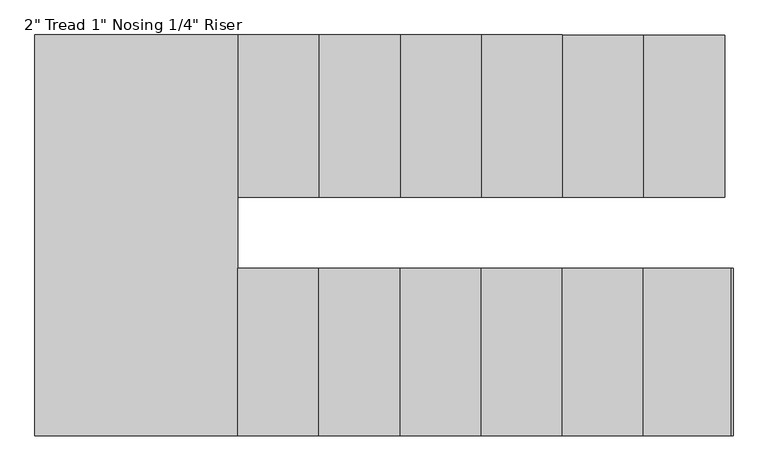
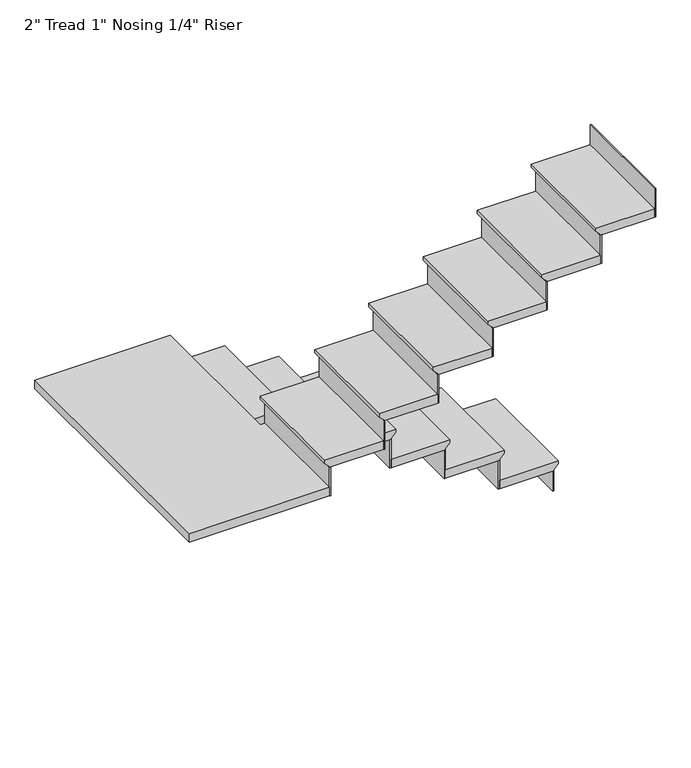
"""IFC4 building model written with IfcOpenShell, lengths in millimetres: stair flight geometry."""

from ifc_helpers import new_model, si_unit, origin, place, context, project, spatial, faceted_brep, source, transform, mapped, element, save


def stair_flight_411a5c89(model_context):
    return source(origin(), model_context, "Body", "Brep", [
        faceted_brep([(-2968.8120155, -2170.0065691, 12951.8833333), (-2968.8120155, -2170.0065691, 12970.9333333), (-2968.8120155, -2779.6065691, 12970.9333333), (-2968.8120155, -2779.6065691, 12951.8833333), (-2994.2120155, -2170.0065691, 12926.4833333), (-2994.2120155, -2779.6065691, 12926.4833333), (-3299.0120155, -2170.0065691, 12970.9333333), (-3299.0120155, -2779.6065691, 12970.9333333), (-2994.2120155, -2779.6065691, 12920.1333333), (-3299.0120155, -2779.6065691, 12920.1333333), (-3299.0120155, -2170.0065691, 12920.1333333), (-2994.2120155, -2170.0065691, 12920.1333333)], [[[0, 1, 2, 3]], [[4, 0, 3, 5]], [[2, 1, 6, 7]], [[8, 9, 10, 11]], [[2, 7, 9, 8, 5, 3]], [[8, 11, 4, 5]], [[6, 1, 0, 4, 11, 10]], [[7, 6, 10, 9]]]),
        faceted_brep([(-2994.2120155, -2170.0065691, 12920.1333333), (-2994.2120155, -2170.0065691, 12801.6), (-3000.5620155, -2170.0065691, 12801.6), (-3000.5620155, -2170.0065691, 12920.1333333), (-2994.2120155, -2779.6065691, 12920.1333333), (-3000.5620155, -2779.6065691, 12920.1333333), (-3000.5620155, -2779.6065691, 12801.6), (-2994.2120155, -2779.6065691, 12801.6)], [[[0, 1, 2, 3]], [[4, 5, 6, 7]], [[1, 0, 4, 7]], [[2, 1, 7, 6]], [[3, 2, 6, 5]], [[0, 3, 5, 4]]]),
        faceted_brep([(-3299.0120155, -2170.0065691, 13089.4666667), (-3299.0120155, -2170.0065691, 12920.1333333), (-3305.3620155, -2170.0065691, 12920.1333333), (-3305.3620155, -2170.0065691, 13089.4666667), (-3299.0120155, -2779.6065691, 13089.4666667), (-3305.3620155, -2779.6065691, 13089.4666667), (-3305.3620155, -2779.6065691, 12920.1333333), (-3299.0120155, -2779.6065691, 12920.1333333)], [[[0, 1, 2, 3]], [[4, 5, 6, 7]], [[1, 0, 4, 7]], [[2, 1, 7, 6]], [[3, 2, 6, 5]], [[0, 3, 5, 4]]]),
        faceted_brep([(-3273.6120155, -2779.6065691, 13140.2666667), (-3273.6120155, -2170.0065691, 13140.2666667), (-3603.8120155, -2170.0065691, 13140.2666667), (-3603.8120155, -2779.6065691, 13140.2666667), (-3299.0120155, -2779.6065691, 13089.4666667), (-3603.8120155, -2779.6065691, 13089.4666667), (-3603.8120155, -2170.0065691, 13089.4666667), (-3299.0120155, -2170.0065691, 13089.4666667), (-3299.0120155, -2779.6065691, 13095.8166667), (-3273.6120155, -2779.6065691, 13121.2166667), (-3299.0120155, -2170.0065691, 13095.8166667), (-3273.6120155, -2170.0065691, 13121.2166667)], [[[0, 1, 2, 3]], [[4, 5, 6, 7]], [[0, 3, 5, 4, 8, 9]], [[4, 7, 10, 8]], [[2, 1, 11, 10, 7, 6]], [[3, 2, 6, 5]], [[11, 1, 0, 9]], [[10, 11, 9, 8]]]),
        faceted_brep([(-3603.8120155, -2170.0065691, 13258.8), (-3603.8120155, -2170.0065691, 13089.4666667), (-3610.1620155, -2170.0065691, 13089.4666667), (-3610.1620155, -2170.0065691, 13258.8), (-3603.8120155, -2779.6065691, 13258.8), (-3610.1620155, -2779.6065691, 13258.8), (-3610.1620155, -2779.6065691, 13089.4666667), (-3603.8120155, -2779.6065691, 13089.4666667)], [[[0, 1, 2, 3]], [[4, 5, 6, 7]], [[1, 0, 4, 7]], [[2, 1, 7, 6]], [[3, 2, 6, 5]], [[0, 3, 5, 4]]]),
        faceted_brep([(-3578.4120155, -2779.6065691, 13309.6), (-3578.4120155, -2170.0065691, 13309.6), (-3908.6120155, -2170.0065691, 13309.6), (-3908.6120155, -2779.6065691, 13309.6), (-3603.8120155, -2779.6065691, 13258.8), (-3908.6120155, -2779.6065691, 13258.8), (-3908.6120155, -2170.0065691, 13258.8), (-3603.8120155, -2170.0065691, 13258.8), (-3603.8120155, -2779.6065691, 13265.15), (-3578.4120155, -2779.6065691, 13290.55), (-3603.8120155, -2170.0065691, 13265.15), (-3578.4120155, -2170.0065691, 13290.55)], [[[0, 1, 2, 3]], [[4, 5, 6, 7]], [[0, 3, 5, 4, 8, 9]], [[4, 7, 10, 8]], [[2, 1, 11, 10, 7, 6]], [[3, 2, 6, 5]], [[11, 1, 0, 9]], [[10, 11, 9, 8]]]),
        faceted_brep([(-3908.6120155, -2170.0065691, 13428.1333333), (-3908.6120155, -2170.0065691, 13258.8), (-3914.9620155, -2170.0065691, 13258.8), (-3914.9620155, -2170.0065691, 13428.1333333), (-3908.6120155, -2779.6065691, 13428.1333333), (-3914.9620155, -2779.6065691, 13428.1333333), (-3914.9620155, -2779.6065691, 13258.8), (-3908.6120155, -2779.6065691, 13258.8)], [[[0, 1, 2, 3]], [[4, 5, 6, 7]], [[1, 0, 4, 7]], [[2, 1, 7, 6]], [[3, 2, 6, 5]], [[0, 3, 5, 4]]]),
        faceted_brep([(-3883.2120155, -2779.6065691, 13478.9333333), (-3883.2120155, -2170.0065691, 13478.9333333), (-4213.4120155, -2170.0065691, 13478.9333333), (-4213.4120155, -2779.6065691, 13478.9333333), (-3908.6120155, -2779.6065691, 13428.1333333), (-4213.4120155, -2779.6065691, 13428.1333333), (-4213.4120155, -2170.0065691, 13428.1333333), (-3908.6120155, -2170.0065691, 13428.1333333), (-3908.6120155, -2779.6065691, 13434.4833333), (-3883.2120155, -2779.6065691, 13459.8833333), (-3908.6120155, -2170.0065691, 13434.4833333), (-3883.2120155, -2170.0065691, 13459.8833333)], [[[0, 1, 2, 3]], [[4, 5, 6, 7]], [[0, 3, 5, 4, 8, 9]], [[4, 7, 10, 8]], [[2, 1, 11, 10, 7, 6]], [[3, 2, 6, 5]], [[11, 1, 0, 9]], [[10, 11, 9, 8]]]),
        faceted_brep([(-4213.4120155, -2170.0065691, 13597.4666667), (-4213.4120155, -2170.0065691, 13428.1333333), (-4219.7620155, -2170.0065691, 13428.1333333), (-4219.7620155, -2170.0065691, 13597.4666667), (-4213.4120155, -2779.6065691, 13597.4666667), (-4219.7620155, -2779.6065691, 13597.4666667), (-4219.7620155, -2779.6065691, 13428.1333333), (-4213.4120155, -2779.6065691, 13428.1333333)], [[[0, 1, 2, 3]], [[4, 5, 6, 7]], [[1, 0, 4, 7]], [[2, 1, 7, 6]], [[3, 2, 6, 5]], [[0, 3, 5, 4]]]),
        faceted_brep([(-4188.0120155, -2779.6065691, 13648.2666667), (-4188.0120155, -2170.0065691, 13648.2666667), (-4518.2120155, -2170.0065691, 13648.2666667), (-4518.2120155, -2779.6065691, 13648.2666667), (-4213.4120155, -2779.6065691, 13597.4666667), (-4518.2120155, -2779.6065691, 13597.4666667), (-4518.2120155, -2170.0065691, 13597.4666667), (-4213.4120155, -2170.0065691, 13597.4666667), (-4213.4120155, -2779.6065691, 13603.8166667), (-4188.0120155, -2779.6065691, 13629.2166667), (-4213.4120155, -2170.0065691, 13603.8166667), (-4188.0120155, -2170.0065691, 13629.2166667)], [[[0, 1, 2, 3]], [[4, 5, 6, 7]], [[0, 3, 5, 4, 8, 9]], [[4, 7, 10, 8]], [[2, 1, 11, 10, 7, 6]], [[3, 2, 6, 5]], [[11, 1, 0, 9]], [[10, 11, 9, 8]]]),
        faceted_brep([(-4518.2120155, -2170.0065691, 13766.8), (-4518.2120155, -2170.0065691, 13597.4666667), (-4524.5620155, -2170.0065691, 13597.4666667), (-4524.5620155, -2170.0065691, 13766.8), (-4518.2120155, -2779.6065691, 13766.8), (-4524.5620155, -2779.6065691, 13766.8), (-4524.5620155, -2779.6065691, 13597.4666667), (-4518.2120155, -2779.6065691, 13597.4666667)], [[[0, 1, 2, 3]], [[4, 5, 6, 7]], [[1, 0, 4, 7]], [[2, 1, 7, 6]], [[3, 2, 6, 5]], [[0, 3, 5, 4]]]),
        faceted_brep([(-4492.8120155, -2779.6065691, 13817.6), (-4492.8120155, -2170.0065691, 13817.6), (-4823.0120155, -2170.0065691, 13817.6), (-4823.0120155, -2779.6065691, 13817.6), (-4518.2120155, -2779.6065691, 13766.8), (-4823.0120155, -2779.6065691, 13766.8), (-4823.0120155, -2170.0065691, 13766.8), (-4518.2120155, -2170.0065691, 13766.8), (-4518.2120155, -2779.6065691, 13773.15), (-4492.8120155, -2779.6065691, 13798.55), (-4518.2120155, -2170.0065691, 13773.15), (-4492.8120155, -2170.0065691, 13798.55)], [[[0, 1, 2, 3]], [[4, 5, 6, 7]], [[0, 3, 5, 4, 8, 9]], [[4, 7, 10, 8]], [[2, 1, 11, 10, 7, 6]], [[3, 2, 6, 5]], [[11, 1, 0, 9]], [[10, 11, 9, 8]]]),
        faceted_brep([(-4823.0120155, -2170.0065691, 13936.1333333), (-4823.0120155, -2170.0065691, 13766.8), (-4829.3620155, -2170.0065691, 13766.8), (-4829.3620155, -2170.0065691, 13936.1333333), (-4823.0120155, -2779.6065691, 13936.1333333), (-4829.3620155, -2779.6065691, 13936.1333333), (-4829.3620155, -2779.6065691, 13766.8), (-4823.0120155, -2779.6065691, 13766.8)], [[[0, 1, 2, 3]], [[4, 5, 6, 7]], [[1, 0, 4, 7]], [[2, 1, 7, 6]], [[3, 2, 6, 5]], [[0, 3, 5, 4]]]),
        faceted_brep([(-4772.2120155, -3046.3065691, 13986.9333333), (-4797.6120155, -3046.3065691, 13986.9333333), (-4797.6120155, -2170.0065691, 13986.9333333), (-5559.6120155, -2170.0065691, 13986.9333333), (-5559.6120155, -3674.9565691, 13986.9333333), (-4772.2120155, -3674.9565691, 13986.9333333), (-4797.6120155, -3046.3065691, 13936.1333333), (-4772.2120155, -3046.3065691, 13936.1333333), (-4772.2120155, -3674.9565691, 13936.1333333), (-5559.6120155, -3674.9565691, 13936.1333333), (-5559.6120155, -2170.0065691, 13936.1333333), (-4823.0120155, -2170.0065691, 13936.1333333), (-4823.0120155, -2779.6065691, 13936.1333333), (-4797.6120155, -2779.6065691, 13936.1333333), (-4797.6120155, -2779.6065691, 13967.8833333), (-4797.6120155, -2170.0065691, 13967.8833333), (-4823.0120155, -2779.6065691, 13942.4833333), (-4823.0120155, -2170.0065691, 13942.4833333)], [[[0, 1, 2, 3, 4, 5]], [[6, 7, 8, 9, 10, 11, 12, 13]], [[1, 0, 7, 6]], [[2, 1, 6, 13, 14, 15]], [[13, 12, 16, 14]], [[12, 11, 17, 16]], [[3, 2, 15, 17, 11, 10]], [[4, 3, 10, 9]], [[5, 4, 9, 8]], [[0, 5, 8, 7]], [[17, 15, 14, 16]]]),
        faceted_brep([(-4772.2120155, -3674.9565691, 14105.4666667), (-4772.2120155, -3674.9565691, 13936.1333333), (-4765.8620155, -3674.9565691, 13936.1333333), (-4765.8620155, -3674.9565691, 14105.4666667), (-4772.2120155, -3046.3065691, 14105.4666667), (-4765.8620155, -3046.3065691, 14105.4666667), (-4765.8620155, -3046.3065691, 13936.1333333), (-4772.2120155, -3046.3065691, 13936.1333333)], [[[0, 1, 2, 3]], [[4, 5, 6, 7]], [[1, 0, 4, 7]], [[2, 1, 7, 6]], [[3, 2, 6, 5]], [[0, 3, 5, 4]]]),
        faceted_brep([(-4797.6120155, -3046.3065691, 14156.2666667), (-4797.6120155, -3674.9565691, 14156.2666667), (-4467.4120155, -3674.9565691, 14156.2666667), (-4467.4120155, -3046.3065691, 14156.2666667), (-4772.2120155, -3046.3065691, 14105.4666667), (-4467.4120155, -3046.3065691, 14105.4666667), (-4467.4120155, -3674.9565691, 14105.4666667), (-4772.2120155, -3674.9565691, 14105.4666667), (-4772.2120155, -3046.3065691, 14111.8166667), (-4797.6120155, -3046.3065691, 14137.2166667), (-4772.2120155, -3674.9565691, 14111.8166667), (-4797.6120155, -3674.9565691, 14137.2166667)], [[[0, 1, 2, 3]], [[4, 5, 6, 7]], [[0, 3, 5, 4, 8, 9]], [[4, 7, 10, 8]], [[2, 1, 11, 10, 7, 6]], [[3, 2, 6, 5]], [[11, 1, 0, 9]], [[10, 11, 9, 8]]]),
        faceted_brep([(-4467.4120155, -3674.9565691, 14274.8), (-4467.4120155, -3674.9565691, 14105.4666667), (-4461.0620155, -3674.9565691, 14105.4666667), (-4461.0620155, -3674.9565691, 14274.8), (-4467.4120155, -3046.3065691, 14274.8), (-4461.0620155, -3046.3065691, 14274.8), (-4461.0620155, -3046.3065691, 14105.4666667), (-4467.4120155, -3046.3065691, 14105.4666667)], [[[0, 1, 2, 3]], [[4, 5, 6, 7]], [[1, 0, 4, 7]], [[2, 1, 7, 6]], [[3, 2, 6, 5]], [[0, 3, 5, 4]]]),
        faceted_brep([(-4492.8120155, -3046.3065691, 14325.6), (-4492.8120155, -3674.9565691, 14325.6), (-4162.6120155, -3674.9565691, 14325.6), (-4162.6120155, -3046.3065691, 14325.6), (-4467.4120155, -3046.3065691, 14274.8), (-4162.6120155, -3046.3065691, 14274.8), (-4162.6120155, -3674.9565691, 14274.8), (-4467.4120155, -3674.9565691, 14274.8), (-4467.4120155, -3046.3065691, 14281.15), (-4492.8120155, -3046.3065691, 14306.55), (-4467.4120155, -3674.9565691, 14281.15), (-4492.8120155, -3674.9565691, 14306.55)], [[[0, 1, 2, 3]], [[4, 5, 6, 7]], [[0, 3, 5, 4, 8, 9]], [[4, 7, 10, 8]], [[2, 1, 11, 10, 7, 6]], [[3, 2, 6, 5]], [[11, 1, 0, 9]], [[10, 11, 9, 8]]]),
        faceted_brep([(-4162.6120155, -3674.9565691, 14444.1333333), (-4162.6120155, -3674.9565691, 14274.8), (-4156.2620155, -3674.9565691, 14274.8), (-4156.2620155, -3674.9565691, 14444.1333333), (-4162.6120155, -3046.3065691, 14444.1333333), (-4156.2620155, -3046.3065691, 14444.1333333), (-4156.2620155, -3046.3065691, 14274.8), (-4162.6120155, -3046.3065691, 14274.8)], [[[0, 1, 2, 3]], [[4, 5, 6, 7]], [[1, 0, 4, 7]], [[2, 1, 7, 6]], [[3, 2, 6, 5]], [[0, 3, 5, 4]]]),
        faceted_brep([(-4188.0120155, -3046.3065691, 14494.9333333), (-4188.0120155, -3674.9565691, 14494.9333333), (-3857.8120155, -3674.9565691, 14494.9333333), (-3857.8120155, -3046.3065691, 14494.9333333), (-4162.6120155, -3046.3065691, 14444.1333333), (-3857.8120155, -3046.3065691, 14444.1333333), (-3857.8120155, -3674.9565691, 14444.1333333), (-4162.6120155, -3674.9565691, 14444.1333333), (-4162.6120155, -3046.3065691, 14450.4833333), (-4188.0120155, -3046.3065691, 14475.8833333), (-4162.6120155, -3674.9565691, 14450.4833333), (-4188.0120155, -3674.9565691, 14475.8833333)], [[[0, 1, 2, 3]], [[4, 5, 6, 7]], [[0, 3, 5, 4, 8, 9]], [[4, 7, 10, 8]], [[2, 1, 11, 10, 7, 6]], [[3, 2, 6, 5]], [[11, 1, 0, 9]], [[10, 11, 9, 8]]]),
        faceted_brep([(-3857.8120155, -3674.9565691, 14613.4666667), (-3857.8120155, -3674.9565691, 14444.1333333), (-3851.4620155, -3674.9565691, 14444.1333333), (-3851.4620155, -3674.9565691, 14613.4666667), (-3857.8120155, -3046.3065691, 14613.4666667), (-3851.4620155, -3046.3065691, 14613.4666667), (-3851.4620155, -3046.3065691, 14444.1333333), (-3857.8120155, -3046.3065691, 14444.1333333)], [[[0, 1, 2, 3]], [[4, 5, 6, 7]], [[1, 0, 4, 7]], [[2, 1, 7, 6]], [[3, 2, 6, 5]], [[0, 3, 5, 4]]]),
        faceted_brep([(-3883.2120155, -3046.3065691, 14664.2666667), (-3883.2120155, -3674.9565691, 14664.2666667), (-3553.0120155, -3674.9565691, 14664.2666667), (-3553.0120155, -3046.3065691, 14664.2666667), (-3857.8120155, -3046.3065691, 14613.4666667), (-3553.0120155, -3046.3065691, 14613.4666667), (-3553.0120155, -3674.9565691, 14613.4666667), (-3857.8120155, -3674.9565691, 14613.4666667), (-3857.8120155, -3046.3065691, 14619.8166667), (-3883.2120155, -3046.3065691, 14645.2166667), (-3857.8120155, -3674.9565691, 14619.8166667), (-3883.2120155, -3674.9565691, 14645.2166667)], [[[0, 1, 2, 3]], [[4, 5, 6, 7]], [[0, 3, 5, 4, 8, 9]], [[4, 7, 10, 8]], [[2, 1, 11, 10, 7, 6]], [[3, 2, 6, 5]], [[11, 1, 0, 9]], [[10, 11, 9, 8]]]),
        faceted_brep([(-3553.0120155, -3674.9565691, 14782.8), (-3553.0120155, -3674.9565691, 14613.4666667), (-3546.6620155, -3674.9565691, 14613.4666667), (-3546.6620155, -3674.9565691, 14782.8), (-3553.0120155, -3046.3065691, 14782.8), (-3546.6620155, -3046.3065691, 14782.8), (-3546.6620155, -3046.3065691, 14613.4666667), (-3553.0120155, -3046.3065691, 14613.4666667)], [[[0, 1, 2, 3]], [[4, 5, 6, 7]], [[1, 0, 4, 7]], [[2, 1, 7, 6]], [[3, 2, 6, 5]], [[0, 3, 5, 4]]]),
        faceted_brep([(-3578.4120155, -3046.3065691, 14833.6), (-3578.4120155, -3674.9565691, 14833.6), (-3248.2120155, -3674.9565691, 14833.6), (-3248.2120155, -3046.3065691, 14833.6), (-3553.0120155, -3046.3065691, 14782.8), (-3248.2120155, -3046.3065691, 14782.8), (-3248.2120155, -3674.9565691, 14782.8), (-3553.0120155, -3674.9565691, 14782.8), (-3553.0120155, -3046.3065691, 14789.15), (-3578.4120155, -3046.3065691, 14814.55), (-3553.0120155, -3674.9565691, 14789.15), (-3578.4120155, -3674.9565691, 14814.55)], [[[0, 1, 2, 3]], [[4, 5, 6, 7]], [[0, 3, 5, 4, 8, 9]], [[4, 7, 10, 8]], [[2, 1, 11, 10, 7, 6]], [[3, 2, 6, 5]], [[11, 1, 0, 9]], [[10, 11, 9, 8]]]),
        faceted_brep([(-3248.2120155, -3674.9565691, 14952.1333333), (-3248.2120155, -3674.9565691, 14782.8), (-3241.8620155, -3674.9565691, 14782.8), (-3241.8620155, -3674.9565691, 14952.1333333), (-3248.2120155, -3046.3065691, 14952.1333333), (-3241.8620155, -3046.3065691, 14952.1333333), (-3241.8620155, -3046.3065691, 14782.8), (-3248.2120155, -3046.3065691, 14782.8)], [[[0, 1, 2, 3]], [[4, 5, 6, 7]], [[1, 0, 4, 7]], [[2, 1, 7, 6]], [[3, 2, 6, 5]], [[0, 3, 5, 4]]]),
        faceted_brep([(-2943.4120155, -3674.9565691, 15121.4666667), (-2943.4120155, -3674.9565691, 14952.1333333), (-2937.0620155, -3674.9565691, 14952.1333333), (-2937.0620155, -3674.9565691, 15121.4666667), (-2943.4120155, -3046.3065691, 15121.4666667), (-2937.0620155, -3046.3065691, 15121.4666667), (-2937.0620155, -3046.3065691, 14952.1333333), (-2943.4120155, -3046.3065691, 14952.1333333)], [[[0, 1, 2, 3]], [[4, 5, 6, 7]], [[1, 0, 4, 7]], [[2, 1, 7, 6]], [[3, 2, 6, 5]], [[0, 3, 5, 4]]]),
        faceted_brep([(-3273.6120155, -3046.3065691, 15002.9333333), (-3273.6120155, -3674.9565691, 15002.9333333), (-2943.4120155, -3674.9565691, 15002.9333333), (-2943.4120155, -3046.3065691, 15002.9333333), (-3248.2120155, -3046.3065691, 14952.1333333), (-2943.4120155, -3046.3065691, 14952.1333333), (-2943.4120155, -3674.9565691, 14952.1333333), (-3248.2120155, -3674.9565691, 14952.1333333), (-3248.2120155, -3046.3065691, 14958.4833333), (-3273.6120155, -3046.3065691, 14983.8833333), (-3248.2120155, -3674.9565691, 14958.4833333), (-3273.6120155, -3674.9565691, 14983.8833333)], [[[0, 1, 2, 3]], [[4, 5, 6, 7]], [[0, 3, 5, 4, 8, 9]], [[4, 7, 10, 8]], [[2, 1, 11, 10, 7, 6]], [[3, 2, 6, 5]], [[11, 1, 0, 9]], [[10, 11, 9, 8]]]),
    ])


if __name__ == "__main__":
    model = new_model("IFC4")
    model_context = context("Model", 3, world=origin())
    ifc_project = project(units=[si_unit("LENGTHUNIT", "METRE", prefix="MILLI")], contexts=[model_context])
    site = spatial("IfcSite", under=ifc_project)
    building = spatial("IfcBuilding", under=site)
    placement = place(None, origin())
    stair_flight_shape = stair_flight_411a5c89(model_context)
    element("IfcStairFlight", 1, ObjectType="2\" Tread 1\" Nosing 1/4\" Riser", at=placement, inside=building, context=model_context, shape_type="MappedRepresentation", body=[
        mapped(stair_flight_shape, transform((0.0, 0.0, 0.0), x_axis=(1.0, 0.0, 0.0), y_axis=(0.0, 1.0, 0.0), z_axis=(0.0, 0.0, 1.0))),
    ])
    save(model, "model.ifc")
